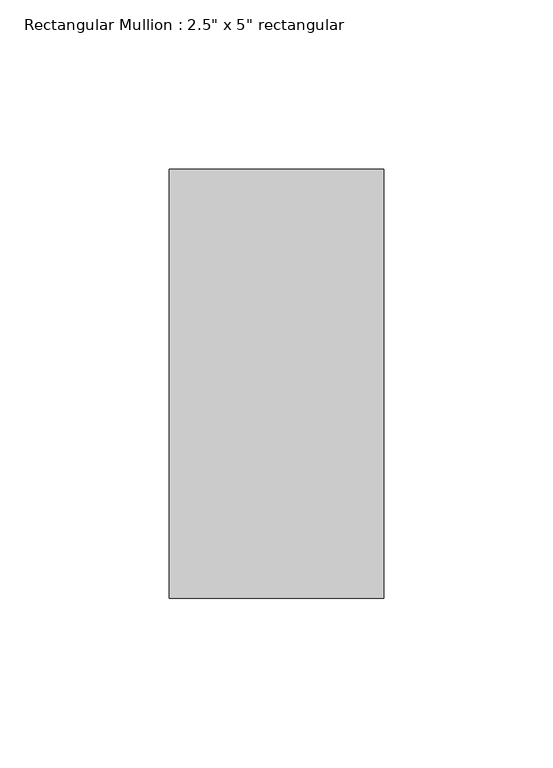
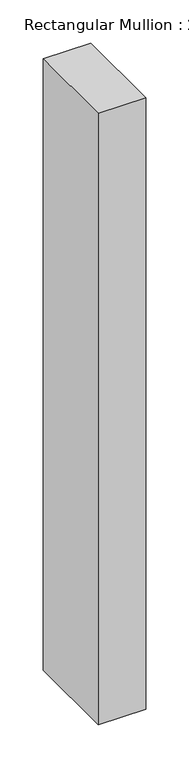
"""IFC4 building model written with IfcOpenShell, lengths in millimetres: member geometry."""

from ifc_helpers import new_model, si_unit, frame, origin, place, context, project, spatial, polyline, outline, extrude, source, transform, mapped, element, save


def member_fd92426f(model_context):
    return source(origin(), model_context, "Body", "SweptSolid", [
        extrude(outline(polyline([(31.75, 63.5), (31.75, -63.5), (-31.75, -63.5), (-31.75, 63.5), (31.75, 63.5)])), frame((0.0, 0.0, -863.6), z_axis=(0.0, 0.0, 1.0), x_axis=(1.0, 0.0, 0.0)), (0.0, 0.0, 1.0), 863.6),
    ])


if __name__ == "__main__":
    model = new_model("IFC4")
    model_context = context("Model", 3, world=origin())
    ifc_project = project(units=[si_unit("LENGTHUNIT", "METRE", prefix="MILLI")], contexts=[model_context])
    site = spatial("IfcSite", under=ifc_project)
    building = spatial("IfcBuilding", under=site)
    placement = place(None, origin())
    member_shape = member_fd92426f(model_context)
    element("IfcMember", 1, ObjectType="Rectangular Mullion : 2.5\" x 5\" rectangular", at=placement, inside=building, context=model_context, shape_type="MappedRepresentation", body=[
        mapped(member_shape, transform((0.0, 0.0, 0.0), x_axis=(1.0, 0.0, 0.0), y_axis=(0.0, 1.0, 0.0), z_axis=(0.0, 0.0, 1.0))),
    ])
    save(model, "model.ifc")

# Revit data of these elements
# Type "Rectangular Mullion : 2.5\" x 5\" rectangular"
#   built-in parameter 1007304 = 0.416667 (stored number, unit not read)
#   built-in parameter 1007301 = 0.104167 (stored number, unit not read)
#   built-in parameter 1007300 = 0.104167 (stored number, unit not read)
# Element 1 (IfcMember, "Rectangular Mullion : 2.5\" x 5\" rectangular")
#   Materials on its faces: "Aluminum"
# Materials
#   "Aluminum": class "Metal", colour RGB 247 247 247, transparency 0, Description = "Aluminum 6061", Cost = 0
